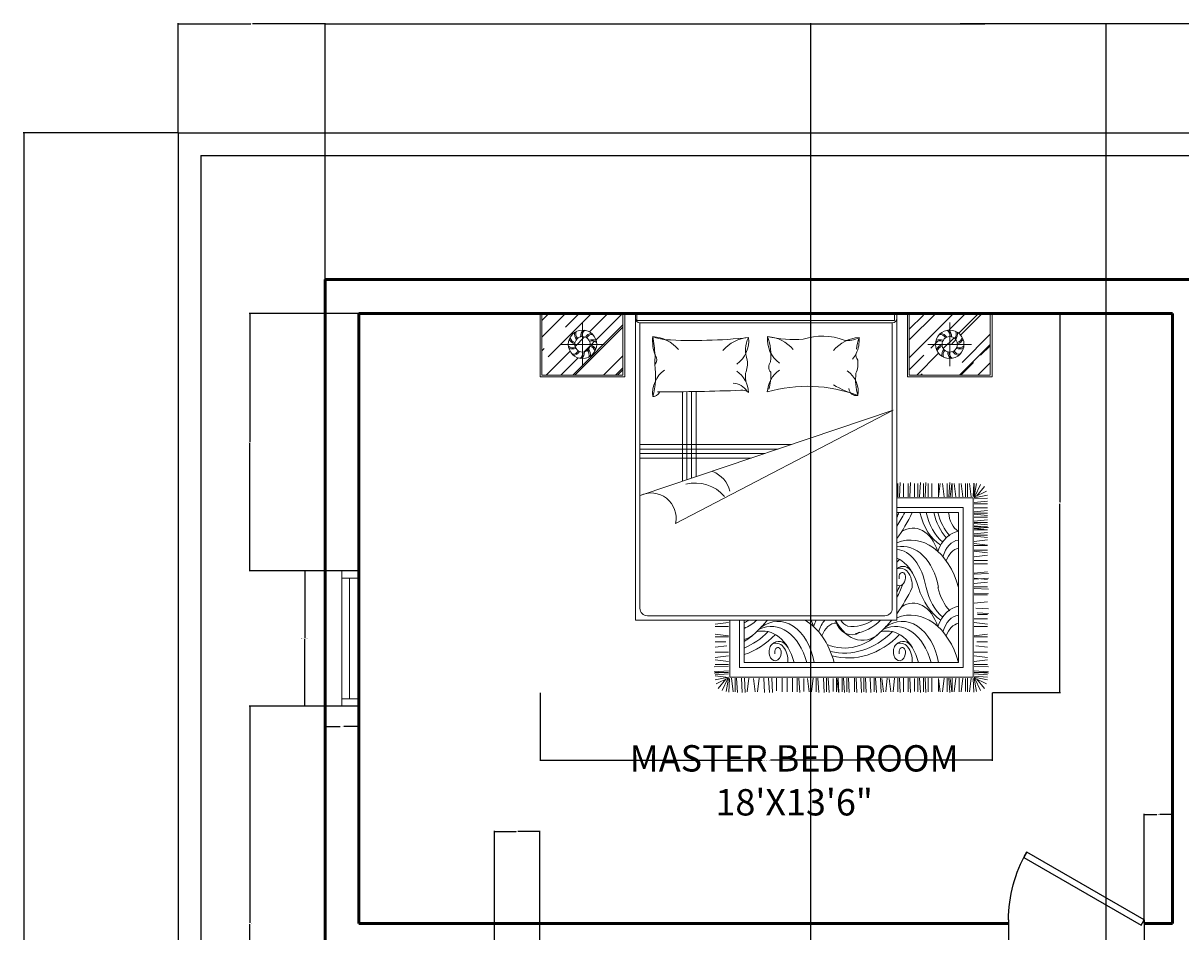
# Model space of a CAD drawing. Units: inches. Extents: x -28 to 483, y -584 to 51.
# Tile 5 of 6: x -28 to 279, y -191 to 51. Entities that reach past the tile are written whole.
import ezdxf

# ---------------------------------------------------------------- set-up
doc = ezdxf.new("R2010")
doc.units = ezdxf.units.IN
doc.header["$MEASUREMENT"] = 0
for name, color, linetype, lineweight in [('A-ANNO-DIMS', 2, 'Continuous', 18), ('A-AREA-IDEN', 7, 'Continuous', 25), ('A-DOOR', 4, 'Continuous', 25), ('A-FURN', 30, 'Continuous', 18), ('A-GLAZ', 5, 'Continuous', 18), ('A-WALL', 7, 'Continuous', 50), ('C-PROP', 7, 'Continuous', 25)]:
    doc.layers.add(name, color=color, linetype=linetype, lineweight=lineweight)
doc.styles.get("Standard").update_dxf_attribs({"font": 'arial.ttf'})
doc.dimstyles.get("Standard").update_dxf_attribs({"dimtxt": 0.18, "dimasz": 0.18, "dimexe": 0.18, "dimexo": 0.0625, "dimgap": 0.09, "dimtad": 0, "dimtih": 1, "dimtoh": 1, "dimdec": 4, "dimzin": 0, "dimdsep": 46, "dimtxsty": 'Standard', "dimcen": 0.09, "dimadec": 0, "dimazin": 0, "dimtfac": 1, "dimtdec": 4, "dimtofl": 0, "dimtmove": 0, "dimatfit": 3, "dimfxl": 1, "dimtolj": 1, "dimtzin": 0, "dimarcsym": 0})

# ---------------------------------------------------------------- blocks, each defined once
blk = doc.blocks.new('*U2')
for p, q in [((0, 0), (0, -6)), ((40, 0), (40, -6))]:
    blk.add_line(p, q)
blk.add_lwpolyline([(0, 0), (34.64, 20), (35.52, 18.48), (0.87, -1.52)], close=True)
blk.add_arc((0, 0), 40, 0, 30)
blk = doc.blocks.new('A$C64B41DC1')
for p, q in [((0, 2.5079), (2.9903, 2.5079)), ((0, 2.0879), (0, 2.5079)), ((0.012, 2.4618), (0.0581, 2.5079)), ((0.012, 2.3515), (0.1684, 2.5079)), ((0.012, 2.0999), (0.012, 2.5079)), ((0.0543, 2.2213), (0.3409, 2.5079)), ((0.1689, 2.4179), (0.2589, 2.5079)), ((0.3265, 2.386), (0.4484, 2.5079)), ((0.3699, 2.3332), (0.5445, 2.5079)), ((0.548, 2.5079), (0.548, 2.0999)), ((0.56, 2.5079), (0.56, 2.0879)), ((0.6301, 2.5079), (0.6301, 0.4779)), ((0.6401, 2.461), (0.6401, 2.5079)), ((0.6401, 2.5079), (2.344, 2.5079)), ((2.344, 2.461), (0.6401, 2.461)), ((2.344, 2.5079), (2.3601, 2.5079)), ((2.344, 2.5079), (2.344, 2.461)), ((2.3601, 2.5079), (2.3601, 2.4761)), ((2.3601, 0.4779), (2.3601, 2.5079)), ((2.4303, 2.5079), (2.4303, 2.0879)), ((2.4423, 2.5079), (2.4423, 2.0999)), ((2.4423, 2.3333), (2.6169, 2.5079)), ((2.4423, 2.2145), (2.7357, 2.5079)), ((2.4423, 2.404), (2.5354, 2.4971)), ((2.705, 2.398), (2.8149, 2.5079)), ((2.7691, 2.3772), (2.8998, 2.5079)), ((2.7819, 2.3646), (2.9252, 2.5079)), ((2.9783, 2.0999), (2.9783, 2.5079)), ((2.9903, 2.0879), (2.9903, 2.5079)), ((0.2157, 2.0999), (0.548, 2.4322)), ((0.2299, 2.0999), (0.548, 2.418)), ((0.2804, 2.1597), (0.2804, 2.4481)), ((0.6601, 2.4461), (1.4951, 2.4461)), ((0.6601, 2.4461), (0.6601, 0.5579)), ((1.4951, 2.4461), (0.6697, 2.4461)), ((2.3301, 2.4461), (1.4951, 2.4461)), ((2.3301, 0.5579), (2.3301, 2.4461)), ((2.7099, 2.1597), (2.7099, 2.4481)), ((0.1362, 2.3039), (0.4246, 2.3039)), ((0.2311, 2.2906), (0.2937, 2.3532)), ((0.3405, 2.3039), (0.3605, 2.3238)), ((2.8541, 2.3039), (2.5657, 2.3039)), ((2.5849, 2.2779), (2.6158, 2.3088)), ((2.6158, 2.3088), (2.6313, 2.3243)), ((2.6674, 2.2756), (2.7382, 2.3464)), ((2.7249, 2.3076), (2.7512, 2.3339)), ((2.7746, 2.0999), (2.9783, 2.3036)), ((2.7914, 2.1846), (2.9783, 2.3715)), ((0.012, 2.261), (0.0275, 2.2765)), ((0.0404, 2.0999), (0.1982, 2.2578)), ((0.2905, 2.2539), (0.3304, 2.2938)), ((0.4194, 2.0999), (0.548, 2.2285)), ((2.4423, 2.1353), (2.5382, 2.2312)), ((2.4918, 2.0999), (2.6366, 2.2447)), ((2.9144, 2.2312), (2.9783, 2.2951)), ((0.1365, 2.0999), (0.251, 2.2144)), ((0.4986, 2.0999), (0.548, 2.1493)), ((2.7831, 2.0999), (2.8678, 2.1846)), ((2.8962, 2.0999), (2.9783, 2.182)), ((0.56, 2.0879), (0, 2.0879)), ((0.548, 2.0999), (0.012, 2.0999)), ((0.5127, 2.0999), (0.548, 2.1352)), ((2.4303, 2.0879), (2.9903, 2.0879)), ((2.4423, 2.0999), (2.9783, 2.0999)), ((2.5172, 2.0999), (2.5269, 2.1096)), ((1.0315, 1.9916), (1.0315, 1.4279)), ((0.9415, 1.9902), (0.9415, 1.3975)), ((0.9715, 1.9906), (0.9715, 1.4076)), ((1.0015, 1.991), (1.0015, 1.4177)), ((2.3349, 1.8678), (0.6613, 1.3029)), ((0.8956, 1.1191), (2.3349, 1.8678)), ((1.6636, 1.6412), (0.6601, 1.6412)), ((1.5748, 1.6112), (0.6601, 1.6112)), ((2.3665, 1.295), (2.3665, 1.3839)), ((2.377, 1.295), (2.3822, 1.3891)), ((2.4032, 1.295), (2.4032, 1.3839)), ((2.4346, 1.295), (2.4346, 1.3839)), ((2.4451, 1.295), (2.4503, 1.3891)), ((2.4774, 1.2957), (2.4774, 1.3837)), ((2.5, 1.295), (2.5, 1.3839)), ((2.5105, 1.295), (2.5157, 1.3891)), ((2.5367, 1.295), (2.5367, 1.3839)), ((2.5471, 1.295), (2.5524, 1.3891)), ((2.5681, 1.295), (2.5681, 1.3839)), ((2.5918, 1.295), (2.5918, 1.3839)), ((2.6346, 1.2957), (2.6346, 1.3837)), ((2.6362, 1.2957), (2.6467, 1.3839)), ((2.6729, 1.295), (2.6624, 1.3839)), ((2.6938, 1.295), (2.6938, 1.3839)), ((2.7043, 1.295), (2.7095, 1.3891)), ((2.7127, 1.2957), (2.7232, 1.3839)), ((2.7253, 1.295), (2.7253, 1.3839)), ((2.7494, 1.295), (2.7389, 1.3839)), ((2.7718, 1.295), (2.7718, 1.3839)), ((2.7959, 1.295), (2.7854, 1.3839)), ((2.8146, 1.2957), (2.8146, 1.3837)), ((2.8146, 1.2957), (2.8146, 1.3837)), ((2.8282, 1.295), (2.8282, 1.3839)), ((2.8282, 1.295), (2.8282, 1.3839)), ((2.8523, 1.295), (2.8418, 1.3839)), ((2.8523, 1.295), (2.8418, 1.3839)), ((2.8653, 1.2966), (2.8688, 1.3861)), ((2.8711, 1.2957), (2.8711, 1.3837)), ((2.8711, 1.2957), (2.8875, 1.3822)), ((2.8713, 1.2927), (2.954, 1.3315)), ((2.8717, 1.2884), (2.9588, 1.3058)), ((2.8765, 1.2958), (2.9132, 1.3758)), ((2.8893, 1.3011), (2.9394, 1.3636)), ((2.3601, 1.2873), (2.8639, 1.2873)), ((2.8639, 1.2873), (2.8639, 0.1018)), ((2.8716, 1.2565), (2.9605, 1.2669)), ((2.8723, 1.2489), (2.9603, 1.2489)), ((2.8744, 1.2817), (2.9603, 1.2869)), ((2.3601, 1.2233), (2.7999, 1.2233)), ((2.3601, 1.1913), (2.7679, 1.1912)), ((2.7679, 1.1912), (2.7679, 0.1978)), ((2.7999, 1.2233), (2.7999, 0.1658)), ((2.8716, 1.2212), (2.9605, 1.2212)), ((2.8716, 1.1947), (2.9605, 1.2052)), ((2.8716, 1.181), (2.9605, 1.1705)), ((2.8716, 1.1595), (2.9605, 1.1595)), ((2.8723, 1.1872), (2.9603, 1.1872)), ((2.8716, 1.133), (2.9605, 1.1435)), ((2.8716, 1.1193), (2.9605, 1.1088)), ((2.8716, 1.1035), (2.9605, 1.093)), ((2.8716, 1.0965), (2.9605, 1.0965)), ((2.8716, 1.086), (2.9657, 1.0913)), ((2.8716, 1.0756), (2.9605, 1.0756)), ((2.8723, 1.1255), (2.9603, 1.1255)), ((2.8723, 1.0858), (2.9605, 1.0753)), ((2.8716, 1.0491), (2.9605, 1.0596)), ((2.8716, 1.0354), (2.9605, 1.0249)), ((2.8723, 1.0416), (2.9603, 1.0416)), ((2.8723, 0.9987), (2.9605, 1.0092)), ((2.8716, 0.9346), (2.9605, 0.9241)), ((2.8723, 0.985), (2.9605, 0.9745)), ((2.8723, 0.9735), (2.9603, 0.9735)), ((2.8723, 0.9408), (2.9603, 0.9408)), ((2.8723, 0.8979), (2.9605, 0.9084)), ((2.8723, 0.8726), (2.9603, 0.8726)), ((2.8723, 0.8505), (2.9603, 0.8505)), ((2.8716, 0.7885), (2.9605, 0.799)), ((2.8716, 0.7818), (2.9657, 0.787)), ((2.8716, 0.7503), (2.9657, 0.7556)), ((2.8716, 0.7204), (2.9605, 0.7309)), ((2.8716, 0.6995), (2.9605, 0.6995)), ((2.8723, 0.7571), (2.9605, 0.7466)), ((2.8716, 0.689), (2.9657, 0.6838)), ((2.8716, 0.6576), (2.9657, 0.6523)), ((2.8716, 0.6471), (2.9605, 0.6471)), ((2.8716, 0.5903), (2.9605, 0.6007)), ((2.882, 0.5582), (2.9657, 0.5536)), ((0.6301, 0.4779), (2.3601, 0.4779)), ((0.7101, 0.5079), (2.2801, 0.5079)), ((1.2465, 0.4625), (1.1576, 0.452)), ((1.2542, 0.1018), (1.2542, 0.4779)), ((1.3182, 0.1658), (1.3182, 0.4779)), ((1.3502, 0.1978), (1.3502, 0.4779)), ((2.8716, 0.4877), (2.9603, 0.4877)), ((2.8716, 0.4625), (2.9605, 0.452)), ((2.8909, 0.5263), (2.9657, 0.5222)), ((2.8928, 0.5169), (2.9605, 0.5169)), ((1.2465, 0.3746), (1.1576, 0.3851)), ((1.2465, 0.4365), (1.1577, 0.4365)), ((2.8716, 0.4365), (2.9603, 0.4365)), ((2.8716, 0.3746), (2.9605, 0.3851)), ((1.2355, 0.3092), (1.1576, 0.3)), ((1.2465, 0.3684), (1.1577, 0.3684)), ((1.2285, 0.3357), (1.1577, 0.3357)), ((2.8716, 0.3684), (2.9603, 0.3684)), ((2.8826, 0.3092), (2.9605, 0.3)), ((2.8896, 0.3357), (2.9603, 0.3357)), ((1.2457, 0.2423), (1.1576, 0.2319)), ((1.2457, 0.2676), (1.1577, 0.2676)), ((2.8723, 0.2676), (2.9603, 0.2676)), ((2.8723, 0.2423), (2.9605, 0.2319)), ((1.2465, 0.1742), (1.1524, 0.169)), ((1.2465, 0.2057), (1.1576, 0.2161)), ((1.2465, 0.1847), (1.1576, 0.1847)), ((2.7999, 0.1658), (1.3182, 0.1658)), ((2.7679, 0.1978), (1.3502, 0.1978)), ((2.8716, 0.2057), (2.9605, 0.2161)), ((2.8716, 0.1847), (2.9605, 0.1847)), ((2.8716, 0.1742), (2.9657, 0.169)), ((1.2465, 0.1428), (1.1524, 0.1376)), ((1.2465, 0.1334), (1.1524, 0.1281)), ((1.2465, 0.1323), (1.1576, 0.1323)), ((1.2465, 0.1323), (1.1576, 0.1323)), ((1.2465, 0.1), (1.1576, 0.1105)), ((1.2465, 0.1229), (1.1588, 0.1168)), ((1.2464, 0.1007), (1.1592, 0.0833)), ((1.2468, 0.0964), (1.1641, 0.0576)), ((1.2288, 0.088), (1.1787, 0.0255)), ((1.2415, 0.0933), (1.2049, 0.0133)), ((1.247, 0.0934), (1.2306, 0.0069)), ((1.2527, 0.0925), (1.2493, 0.003)), ((2.8639, 0.1018), (1.2542, 0.1018)), ((1.2658, 0.0941), (1.2762, 0.0052)), ((1.2899, 0.0941), (1.2899, 0.0052)), ((1.2999, 0.0941), (1.3051, 0)), ((1.3313, 0.0941), (1.3365, 0)), ((1.3523, 0.0941), (1.3575, 0)), ((1.3804, 0.0941), (1.3699, 0.0052)), ((1.4119, 0.0934), (1.4223, 0.0052)), ((1.4485, 0.0941), (1.438, 0.0052)), ((1.48, 0.0941), (1.4852, 0)), ((1.5114, 0.0941), (1.5166, 0)), ((1.5323, 0.0941), (1.5376, 0)), ((1.5638, 0.0941), (1.5638, 0.0105)), ((1.6021, 0.0941), (1.6021, 0.0052)), ((1.6336, 0.0941), (1.6336, 0.0052)), ((1.6702, 0.0941), (1.6702, 0.0052)), ((1.7017, 0.0941), (1.7017, 0.0052)), ((1.7122, 0.0941), (1.7174, 0)), ((1.7445, 0.0934), (1.7445, 0.0054)), ((1.7698, 0.0934), (1.7803, 0.0052)), ((1.8065, 0.0941), (1.796, 0.0052)), ((1.8274, 0.0941), (1.8274, 0.0052)), ((1.8379, 0.0941), (1.8431, 0)), ((1.8746, 0.0941), (1.8798, 0)), ((1.8955, 0.0941), (1.8955, 0.0052)), ((1.906, 0.0941), (1.9113, 0)), ((1.9384, 0.0934), (1.9384, 0.0054)), ((1.9609, 0.0941), (1.9609, 0.0052)), ((1.9636, 0.0934), (1.9741, 0.0052)), ((1.9714, 0.0941), (1.9766, 0)), ((1.9976, 0.0941), (1.9976, 0.0052)), ((2.0081, 0.0941), (2.0133, 0)), ((2.029, 0.0941), (2.029, 0.0052)), ((2.0395, 0.0941), (2.0447, 0)), ((2.0797, 0.0941), (2.0797, 0.0052)), ((2.0902, 0.0941), (2.0954, 0)), ((2.1216, 0.0941), (2.1269, 0)), ((2.1412, 0.0941), (2.1412, 0.0052)), ((2.1517, 0.0941), (2.1569, 0)), ((2.1831, 0.0941), (2.1884, 0)), ((2.2093, 0.0941), (2.2093, 0.0052)), ((2.2198, 0.0941), (2.225, 0)), ((2.2512, 0.0941), (2.2565, 0)), ((2.2603, 0.0934), (2.2707, 0.0052)), ((2.2969, 0.0941), (2.2864, 0.0052)), ((2.3089, 0.0934), (2.3193, 0.0052)), ((2.3455, 0.0941), (2.3351, 0.0052)), ((2.3665, 0.0941), (2.3665, 0.0052)), ((2.377, 0.0941), (2.3822, 0)), ((2.4032, 0.0941), (2.4032, 0.0052)), ((2.4346, 0.0941), (2.4346, 0.0052)), ((2.4451, 0.0941), (2.4503, 0)), ((2.4774, 0.0934), (2.4774, 0.0054)), ((2.5, 0.0941), (2.5, 0.0052)), ((2.5105, 0.0941), (2.5157, 0)), ((2.5367, 0.0941), (2.5367, 0.0052)), ((2.5471, 0.0941), (2.5524, 0)), ((2.5681, 0.0941), (2.5681, 0.0052)), ((2.5918, 0.0941), (2.5918, 0.0052)), ((2.6346, 0.0934), (2.6346, 0.0054)), ((2.6362, 0.0934), (2.6467, 0.0052)), ((2.6729, 0.0941), (2.6624, 0.0052)), ((2.6938, 0.0941), (2.6938, 0.0052)), ((2.7043, 0.0941), (2.7095, 0)), ((2.7127, 0.0934), (2.7232, 0.0052)), ((2.7253, 0.0941), (2.7253, 0.0052)), ((2.7494, 0.0941), (2.7389, 0.0052)), ((2.7718, 0.0941), (2.7718, 0.0052)), ((2.7959, 0.0941), (2.7854, 0.0052)), ((2.8146, 0.0934), (2.8146, 0.0054)), ((2.8282, 0.0941), (2.8282, 0.0052)), ((2.8523, 0.0941), (2.8418, 0.0052)), ((2.8653, 0.0925), (2.8688, 0.003)), ((2.8711, 0.0934), (2.8875, 0.0069)), ((2.8713, 0.0964), (2.954, 0.0576)), ((2.8716, 0.1428), (2.9657, 0.1376)), ((2.8716, 0.1334), (2.9657, 0.1281)), ((2.8716, 0.1323), (2.9605, 0.1323)), ((2.8716, 0.1229), (2.9593, 0.1168)), ((2.8717, 0.1007), (2.9588, 0.0833)), ((2.8744, 0.1074), (2.9603, 0.1022)), ((2.8765, 0.0933), (2.9132, 0.0133)), ((2.8893, 0.088), (2.9394, 0.0255))]:
    blk.add_line(p, q)
at = {"ltscale": 10}
for p, q in [((1.4859, 1.5812), (0.6601, 1.5812)), ((1.397, 1.5512), (0.6601, 1.5512))]:
    blk.add_line(p, q, dxfattribs=at)
for centre, radius in [((0.2804, 2.3039), 0.0942), ((2.7099, 2.3039), 0.0942), ((0.2804, 2.3039), 0.051), ((2.7099, 2.3039), 0.051)]:
    blk.add_circle(centre, radius)
for centre, radius, start, end in [((0.6601, 2.4761), 0.03, 180, 270), ((2.3301, 2.4761), 0.03, 270, 0), ((0.2887, 2.3745), 0.0605, 172.17003, 218.48975), ((0.2828, 2.3731), 0.0462, 160.30017, 220.53802), ((0.3286, 2.3561), 0.0605, 136.17003, 182.48975), ((0.3231, 2.3585), 0.0462, 124.30017, 184.53802), ((0.3501, 2.3178), 0.0605, 100.17003, 146.48975), ((2.6402, 2.3178), 0.0605, 33.51025, 79.82997), ((2.6672, 2.3585), 0.0462, 355.46198, 55.69983), ((2.6617, 2.3561), 0.0605, 357.51025, 43.82997), ((2.7075, 2.3731), 0.0462, 319.46198, 19.69983), ((2.7016, 2.3745), 0.0605, 321.51025, 7.82997), ((0.2457, 2.3659), 0.0605, 208.17003, 254.48975), ((0.2417, 2.3614), 0.0462, 196.30017, 256.53802), ((0.347, 2.323), 0.0462, 88.30017, 148.53802), ((0.3449, 2.2742), 0.0605, 64.17003, 110.48975), ((0.3455, 2.2802), 0.0462, 52.30017, 112.53802), ((0.3151, 2.2419), 0.0605, 28.17003, 74.48975), ((1.0526, 2.3302), 0.3085, 175.30484, 198.69419), ((-0.8702, 2.0941), 1.6364, 4.80985, 9.18918), ((0.8579, 2.6278), 0.2948, 247.51785, 264.26696), ((0.728, 2.111), 0.245, 40.4189, 85.9871), ((1.0164, 5.7096), 3.3803, 266.81337, 276.16021), ((1.3963, 2.1044), 0.245, 94.0129, 139.5811), ((1.1858, 2.3288), 0.1943, 306.5711, 5.88998), ((1.5348, 2.2652), 0.1767, 151.77364, 201.69827), ((1.6986, 2.3355), 0.1943, 174.11002, 233.4289), ((1.1481, 2.2311), 0.3783, 353.49469, 19.18669), ((1.6871, 3.192), 0.8561, 257.74383, 273.62843), ((1.4882, 2.111), 0.245, 40.4189, 85.9871), ((1.8674, 1.9709), 0.3878, 68.20259, 108.9817), ((2.1269, 2.1044), 0.245, 94.0129, 139.5811), ((2.0342, 2.4856), 0.1563, 261.59582, 298.90918), ((1.9165, 2.3288), 0.1943, 333.73715, 5.88998), ((2.6058, 2.2028), 0.517, 163.60457, 172.3273), ((2.6448, 2.2802), 0.0462, 67.46198, 127.69983), ((2.6454, 2.2742), 0.0605, 69.51025, 115.82997), ((2.6752, 2.2419), 0.0605, 105.51025, 151.82997), ((2.6433, 2.323), 0.0462, 31.46198, 91.69983), ((2.7486, 2.3614), 0.0462, 283.46198, 343.69983), ((2.7446, 2.3659), 0.0605, 285.51025, 331.82997), ((0.2153, 2.3276), 0.0462, 232.30017, 292.53802), ((0.2158, 2.3336), 0.0605, 244.17003, 290.48975), ((0.2138, 2.2848), 0.0462, 268.30017, 328.53802), ((0.2107, 2.29), 0.0605, 280.17003, 326.48975), ((0.2377, 2.2493), 0.0462, 304.30017, 4.53802), ((0.2322, 2.2517), 0.0605, 316.17003, 2.48975), ((0.2779, 2.2347), 0.0462, 340.30017, 40.53802), ((0.272, 2.2333), 0.0605, 352.17003, 38.48975), ((0.3191, 2.2464), 0.0462, 16.30017, 76.53802), ((0.7274, 2.2013), 0.0446, 314.4736, 42.17134), ((-1.6008, 2.277), 2.3618, 357.39054, 358.88764), ((1.9165, 2.3288), 0.1943, 320.94042, 333.73715), ((2.1347, 2.2313), 0.0459, 165.35061, 223.26844), ((2.6712, 2.2464), 0.0462, 103.46198, 163.69983), ((2.7182, 2.2333), 0.0605, 141.51025, 187.82997), ((2.7123, 2.2347), 0.0462, 139.46198, 199.69983), ((2.7581, 2.2517), 0.0605, 177.51025, 223.82997), ((2.7526, 2.2493), 0.0462, 175.46198, 235.69983), ((2.7796, 2.29), 0.0605, 213.51025, 259.82997), ((2.7765, 2.2848), 0.0462, 211.46198, 271.69983), ((2.7744, 2.3336), 0.0605, 249.51025, 295.82997), ((2.775, 2.3276), 0.0462, 247.46198, 307.69983), ((0.2688, 2.0945), 0.4956, 344.0243, 8.70709), ((1.204, 2.1778), 0.1681, 337.01697, 7.53676), ((1.5671, 2.1546), 0.0547, 142.08329, 220.902), ((1.9346, 2.1778), 0.1681, 337.01697, 7.53676), ((0.9385, 1.978), 0.1943, 126.5711, 185.88998), ((1.1858, 1.9714), 0.1943, 4.31813, 53.4289), ((1.5415, 2.0969), 0.1834, 175.22328, 196.23004), ((1.7059, 1.9714), 0.204, 127.11975, 175.09005), ((1.1965, 2.0983), 0.3299, 343.79543, 3.55541), ((1.9394, 1.991), 0.1651, 351.26213, 55.75721), ((2.4617, 2.0719), 0.3745, 173.82958, 196.4356), ((0.7246, 18.8439), 16.8552, 270.17399, 272.05214), ((1.2687, 1.9248), 0.1223, 33.62799, 86.47438), ((1.3401, 1.9404), 0.0603, 49.09906, 101.37023), ((1.7676, 1.0629), 0.9631, 69.65065, 105.96307), ((2.2748, 2.5795), 0.6373, 238.34989, 254.31375), ((2.0911, 2.0123), 0.0478, 179.77267, 283.80184), ((0.7417, 2.0149), 0.057, 273.47085, 328.54118), ((0.728, 2.2025), 0.245, 274.0129, 278.34166), ((1.0747, 1.2871), 0.1871, 14.1863, 69.12121), ((1.0274, 1.1334), 0.2527, 40.62904, 104.37123), ((0.7347, 1.1553), 0.1649, 347.31088, 116.44537), ((0.7101, 0.5579), 0.05, 180, 270), ((2.2801, 0.5579), 0.05, 270, 0)]:
    blk.add_arc(centre, radius, start, end)
for centre, major_axis, ratio, start_param, end_param in [((1.9938, 1.6262), (0, -0.7531), 0.68, 0.797284, 0.954936), ((2.0643, 1.466), (0, -0.5322), 0.68, 7.239912, 7.311536), ((1.9052, 1.7397), (0, -0.9842), 0.68, 0.74745, 0.979724), ((2.7455, 1.3081), (0, 0.3614), 0.68, 1.900046, 2.742661), ((2.7868, 1.3081), (0, 0.3614), 0.68, 1.900046, 2.614747), ((2.8372, 1.3081), (0, 0.3614), 0.68, 1.900046, 2.479658), ((2.8607, 1.3211), (0, 0.3614), 0.68, 1.938265, 2.479658), ((2.8057, 1.2079), (0, -0.1524), 0.68, 4.821745, 5.895886), ((2.4665, 0.8216), (0, -0.2664), 0.68, 2.006169, 3.565187), ((2.4513, 0.5069), (0, 0.502), 0.68, 5.095327, 6.553458), ((2.7862, 0.8069), (0, -0.2615), 0.68, 3.244645, 4.205018), ((2.7784, 0.8289), (0, -0.1802), 0.68, 3.227058, 4.318474), ((2.396, 0.6032), (0, 0.3641), 0.68, -1.3172, 0.145284), ((2.3507, 0.5642), (0.0073, 0.3819), 0.56205, -1.21172, -0.009991), ((2.7821, 0.7971), (0, -0.1589), 0.68, 3.272942, 4.229533), ((2.2964, 0.5771), (0, -0.3263), 0.68, 1.938944, 2.850232), ((2.0403, 1.6015), (0, -0.8763), 0.68, 6.849801, 6.887077), ((2.4005, 0.7132), (0, -0.1214), 0.68, 2.284368, 3.652258), ((2.3834, 0.7081), (0, 0.1147), 0.68, 4.593909, 6.585576), ((2.3961, 0.7628), (0, -0.0317), 0.68, 1.462497, 5.046281), ((2.3774, 0.7653), (0, -0.0593), 0.68, 5.841311, 7.755362), ((1.9938, 1.1295), (-0.0678, 0.7439), 0.610498, 3.917146, 4.063997), ((2.0643, 0.9693), (0, -0.5322), 0.68, 7.239912, 7.336618), ((1.9052, 1.243), (0, -0.9842), 0.68, 0.74745, 0.979724), ((2.7455, 0.8114), (-0.0599, 0.3735), 0.695517, 1.775813, 2.548612), ((2.7868, 0.8114), (0, 0.3614), 0.68, 1.900046, 2.614747), ((2.8607, 0.8243), (0, 0.3614), 0.68, 1.938265, 2.479658), ((2.4665, 0.3249), (0, -0.2664), 0.68, 2.006169, 3.565187), ((2.4513, 0.0102), (0, 0.502), 0.68, 5.095327, 6.553458), ((2.7862, 0.3102), (0, -0.2615), 0.68, 3.244645, 4.205018), ((1.242, 0.9693), (0, -0.5322), 0.68, 6.586764, 6.677612), ((1.1714, 1.1295), (-0.1157, 0.7241), 0.59432, 3.291697, 3.50733), ((1.0828, 1.243), (0, -0.9842), 0.68, 0.565948, 0.680366), ((1.5283, 0.0674), (0, -0.3703), 0.68, 1.930561, 3.464283), ((1.5736, 0.1065), (0, 0.3641), 0.68, -1.3172, 0.476403), ((1.6289, 0.0102), (0, 0.502), 0.68, 6.655152, 6.661293), ((1.6289, 0.0102), (0, 0.502), 0.68, 5.095327, 5.911219), ((1.6442, 0.3249), (0, -0.2664), 0.68, 2.006169, 2.182797), ((1.9638, 0.3102), (0, -0.2615), 0.68, 4.015924, 4.205018), ((1.956, 0.3322), (0, -0.1802), 0.68, 3.770744, 4.318474), ((2.0606, 0.5616), (0, -0.1803), 0.68, 5.194792, 5.929328), ((2.0606, 0.5616), (0, -0.1803), 0.68, 5.194792, 6.723255), ((2.1315, 0.6603), (0, -0.3155), 0.68, 5.328638, 6.949396), ((2.0549, 0.5656), (0, -0.1303), 0.68, 5.450951, 6.054641), ((2.0643, 0.9693), (0, -0.5322), 0.68, 6.20013, 6.677612), ((1.9938, 1.1295), (-0.0678, 0.7439), 0.610498, 3.199135, 3.592282), ((1.9052, 1.243), (0, -0.9842), 0.68, 0.565948, 0.680366), ((2.3507, 0.0674), (0, -0.3703), 0.68, 1.930561, 3.464283), ((2.396, 0.1065), (0, 0.3641), 0.68, -1.3172, 0.476403), ((2.4513, 0.0102), (0, 0.502), 0.68, 6.655152, 6.661293), ((2.7784, 0.3322), (0, -0.1802), 0.68, 3.227058, 4.318474), ((1.1933, 0.9181), (0, -0.624), 0.68, 0.378672, 0.625379), ((1.3091, 0.6603), (0, -0.3155), 0.68, 6.475719, 6.949396), ((1.1911, 1.1066), (0, 0.8458), 0.68, 3.421828, 3.728616), ((1.2179, 1.1047), (0, -0.8763), 0.68, 6.507006, 6.887077), ((1.474, 0.0804), (0, -0.3263), 0.68, 1.938944, 3.339184), ((1.9597, 0.3004), (0, -0.1589), 0.68, 3.14258, 4.229533), ((2.0157, 0.9181), (0, -0.624), 0.68, -0.280078, 0.625379), ((2.0135, 1.1066), (0, 0.8458), 0.68, 2.978727, 3.728616), ((2.0403, 1.1047), (0, -0.8763), 0.68, 6.099302, 6.887077), ((2.2964, 0.0804), (0, -0.3263), 0.68, 1.938944, 3.339184), ((2.7821, 0.3004), (0, -0.1589), 0.68, 3.272942, 4.229533), ((1.555, 0.2685), (0, -0.0593), 0.68, 3.732151, 7.755362), ((1.5781, 0.2165), (0, -0.1214), 0.68, 2.284368, 3.726131), ((1.561, 0.2114), (0, 0.1147), 0.68, 4.593909, 6.647252), ((2.3774, 0.2685), (0, -0.0593), 0.68, 3.732151, 7.755362), ((2.4005, 0.2165), (0, -0.1214), 0.68, 2.284368, 3.726131), ((2.3834, 0.2114), (0, 0.1147), 0.68, 4.593909, 6.647252), ((1.5737, 0.2661), (0, -0.0317), 0.68, 1.462497, 5.046281), ((2.3961, 0.2661), (0, -0.0317), 0.68, 1.462497, 5.046281)]:
    blk.add_ellipse(centre, major_axis=major_axis, ratio=ratio, start_param=start_param, end_param=end_param)
blk = doc.blocks.new('WIN-36IN')
for p, q in [((0, 9), (0, 0)), ((2, 9), (2, 4.5)), ((34, 6.5), (2, 6.5)), ((34, 9), (34, 4.5)), ((36, 9), (36, 0)), ((36, 4.5), (0, 4.5))]:
    blk.add_line(p, q)
blk = doc.blocks.new('*D11')
at = {"layer": 'A-ANNO-DIMS', "color": 0, "lineweight": -2, "transparency": 16777216}
for p, q in [((51.78, -94.91), (46.26, -94.91)), ((46.44, -95.09), (46.44, -112.72)), ((46.44, -130.73), (46.44, -113.09)), ((51.78, -130.91), (46.26, -130.91))]:
    blk.add_line(p, q, dxfattribs=at)
at = {"layer": 'A-ANNO-DIMS', "color": 0, "transparency": 16777216}
for points in [[(46.41, -95.09), (46.47, -95.09), (46.44, -94.91)], [(46.41, -130.73), (46.47, -130.73), (46.44, -130.91)]]:
    blk.add_solid(points, dxfattribs=at)
at = {"layer": 'Defpoints', "color": 0, "transparency": 16777216}
for p in [(51.84, -94.91), (46.44, -130.91), (51.84, -130.91)]:
    blk.add_point(p, dxfattribs=at)
at = {"layer": 'A-ANNO-DIMS', "color": 0, "transparency": 16777216, "insert": (46.44, -112.91), "char_height": 0.18, "attachment_point": 5}
blk.add_mtext('\\A1;WINDOW 36 TYP.', dxfattribs=at)
blk = doc.blocks.new('*D12')
at = {"layer": 'A-ANNO-DIMS', "color": 0, "lineweight": -2, "transparency": 16777216}
for p, q in [((51.84, -130.97), (51.84, -136.49)), ((60.84, -130.97), (60.84, -136.49)), ((52.02, -136.31), (55.88, -136.31)), ((60.66, -136.31), (56.8, -136.31))]:
    blk.add_line(p, q, dxfattribs=at)
at = {"layer": 'A-ANNO-DIMS', "color": 0, "transparency": 16777216}
for points in [[(52.02, -136.28), (52.02, -136.34), (51.84, -136.31)], [(60.66, -136.28), (60.66, -136.34), (60.84, -136.31)]]:
    blk.add_solid(points, dxfattribs=at)
at = {"layer": 'Defpoints', "color": 0, "transparency": 16777216}
for p in [(51.84, -130.91), (60.84, -130.91), (60.84, -136.31)]:
    blk.add_point(p, dxfattribs=at)
at = {"layer": 'A-ANNO-DIMS', "color": 0, "transparency": 16777216, "insert": (56.34, -136.31), "char_height": 0.18, "attachment_point": 5}
blk.add_mtext('\\A1;9 TYP.', dxfattribs=at)
blk = doc.blocks.new('*D13')
at = {"layer": 'A-ANNO-DIMS', "color": 0, "lineweight": -2, "transparency": 16777216}
for p, q in [((108.96, -127.31), (108.96, -145.43)), ((228.98, -127.31), (228.98, -145.43)), ((109.14, -145.25), (167.8, -145.25)), ((228.8, -145.25), (170.13, -145.25))]:
    blk.add_line(p, q, dxfattribs=at)
at = {"layer": 'A-ANNO-DIMS', "color": 0, "transparency": 16777216}
for points in [[(109.14, -145.22), (109.14, -145.28), (108.96, -145.25)], [(228.8, -145.22), (228.8, -145.28), (228.98, -145.25)]]:
    blk.add_solid(points, dxfattribs=at)
at = {"layer": 'Defpoints', "color": 0, "transparency": 16777216}
for p in [(108.96, -127.25), (228.98, -127.25), (228.98, -145.25)]:
    blk.add_point(p, dxfattribs=at)
at = {"layer": 'A-ANNO-DIMS', "color": 0, "transparency": 16777216, "insert": (168.97, -145.25), "char_height": 0.18, "attachment_point": 5}
blk.add_mtext('\\A1;BED SET 120 TYP.', dxfattribs=at)
blk = doc.blocks.new('*D14')
at = {"layer": 'A-ANNO-DIMS', "color": 0, "lineweight": -2, "transparency": 16777216}
for p, q in [((229.04, -26.59), (247.16, -26.59)), ((246.98, -26.77), (246.98, -76.74)), ((246.98, -127.07), (246.98, -77.1)), ((229.04, -127.25), (247.16, -127.25))]:
    blk.add_line(p, q, dxfattribs=at)
at = {"layer": 'A-ANNO-DIMS', "color": 0, "transparency": 16777216}
for points in [[(246.95, -26.77), (247.01, -26.77), (246.98, -26.59)], [(246.95, -127.07), (247.01, -127.07), (246.98, -127.25)]]:
    blk.add_solid(points, dxfattribs=at)
at = {"layer": 'Defpoints', "color": 0, "transparency": 16777216}
for p in [(228.98, -26.59), (246.98, -26.59), (228.98, -127.25)]:
    blk.add_point(p, dxfattribs=at)
at = {"layer": 'A-ANNO-DIMS', "color": 0, "transparency": 16777216, "insert": (246.98, -76.92), "char_height": 0.18, "attachment_point": 5}
blk.add_mtext('\\A1;101 TYP.', dxfattribs=at)
blk = doc.blocks.new('*D20')
at = {"layer": 'A-ANNO-DIMS', "color": 0, "lineweight": -2, "transparency": 16777216}
for p, q in [((12.78, 21.41), (-28.29, 21.41)), ((-28.11, 21.23), (-28.11, -266.41)), ((-28.11, -554.41), (-28.11, -266.77)), ((12.78, -554.59), (-28.29, -554.59))]:
    blk.add_line(p, q, dxfattribs=at)
at = {"layer": 'A-ANNO-DIMS', "color": 0, "transparency": 16777216}
for points in [[(-28.14, 21.23), (-28.08, 21.23), (-28.11, 21.41)], [(-28.14, -554.41), (-28.08, -554.41), (-28.11, -554.59)]]:
    blk.add_solid(points, dxfattribs=at)
at = {"layer": 'Defpoints', "color": 0, "transparency": 16777216}
for p in [(-28.11, 21.41), (12.84, 21.41), (12.84, -554.59)]:
    blk.add_point(p, dxfattribs=at)
at = {"layer": 'A-ANNO-DIMS', "color": 0, "transparency": 16777216, "insert": (-28.11, -266.59), "char_height": 0.18, "attachment_point": 5}
blk.add_mtext('\\A1;576', dxfattribs=at)
blk = doc.blocks.new('*D21')
at = {"layer": 'A-ANNO-DIMS', "color": 0, "lineweight": -2, "transparency": 16777216}
for p, q in [((51.84, -17.53), (51.84, 50.54)), ((52.02, 50.36), (227.07, 50.36)), ((402.66, 50.36), (227.61, 50.36)), ((402.84, -17.53), (402.84, 50.54))]:
    blk.add_line(p, q, dxfattribs=at)
at = {"layer": 'A-ANNO-DIMS', "color": 0, "transparency": 16777216}
for points in [[(52.02, 50.39), (52.02, 50.33), (51.84, 50.36)], [(402.66, 50.39), (402.66, 50.33), (402.84, 50.36)]]:
    blk.add_solid(points, dxfattribs=at)
at = {"layer": 'Defpoints', "color": 0, "transparency": 16777216}
for p in [(402.84, 50.36), (51.84, -17.59), (402.84, -17.59)]:
    blk.add_point(p, dxfattribs=at)
at = {"layer": 'A-ANNO-DIMS', "color": 0, "transparency": 16777216, "insert": (227.34, 50.36), "char_height": 0.18, "attachment_point": 5}
blk.add_mtext('\\A1;351', dxfattribs=at)
blk = doc.blocks.new('*D23')
at = {"layer": 'A-ANNO-DIMS', "color": 0, "lineweight": -2, "transparency": 16777216}
for p, q in [((12.84, 21.47), (12.84, 50.54)), ((13.02, 50.36), (32.12, 50.36)), ((51.66, 50.36), (32.56, 50.36)), ((51.84, -17.53), (51.84, 50.54))]:
    blk.add_line(p, q, dxfattribs=at)
at = {"layer": 'A-ANNO-DIMS', "color": 0, "transparency": 16777216}
for points in [[(13.02, 50.39), (13.02, 50.33), (12.84, 50.36)], [(51.66, 50.39), (51.66, 50.33), (51.84, 50.36)]]:
    blk.add_solid(points, dxfattribs=at)
at = {"layer": 'Defpoints', "color": 0, "transparency": 16777216}
for p in [(51.84, 50.36), (12.84, 21.41), (51.84, -17.59)]:
    blk.add_point(p, dxfattribs=at)
at = {"layer": 'A-ANNO-DIMS', "color": 0, "transparency": 16777216, "insert": (32.34, 50.36), "char_height": 0.18, "attachment_point": 5}
blk.add_mtext('\\A1;39', dxfattribs=at)
blk = doc.blocks.new('*D29')
at = {"layer": 'A-ANNO-DIMS', "color": 0, "lineweight": -2, "transparency": 16777216}
for p, q in [((269.35, -188.53), (269.35, -159.46)), ((269.53, -159.64), (272.72, -159.64)), ((276.66, -159.64), (273.47, -159.64)), ((276.84, -188.53), (276.84, -159.46))]:
    blk.add_line(p, q, dxfattribs=at)
at = {"layer": 'A-ANNO-DIMS', "color": 0, "transparency": 16777216}
for points in [[(269.53, -159.61), (269.53, -159.67), (269.35, -159.64)], [(276.66, -159.61), (276.66, -159.67), (276.84, -159.64)]]:
    blk.add_solid(points, dxfattribs=at)
at = {"layer": 'Defpoints', "color": 0, "transparency": 16777216}
for p in [(276.84, -159.64), (269.35, -188.59), (276.84, -188.59)]:
    blk.add_point(p, dxfattribs=at)
at = {"layer": 'A-ANNO-DIMS', "color": 0, "transparency": 16777216, "insert": (273.1, -159.64), "char_height": 0.18, "attachment_point": 5}
blk.add_mtext('\\A1;7.491', dxfattribs=at)
blk = doc.blocks.new('*D33')
at = {"layer": 'A-ANNO-DIMS', "color": 0, "lineweight": -2, "transparency": 16777216}
for p, q in [((60.78, -26.59), (31.71, -26.59)), ((31.89, -26.77), (31.89, -60.57)), ((31.89, -94.73), (31.89, -60.93)), ((60.78, -94.91), (31.71, -94.91))]:
    blk.add_line(p, q, dxfattribs=at)
at = {"layer": 'A-ANNO-DIMS', "color": 0, "transparency": 16777216}
for points in [[(31.86, -26.77), (31.92, -26.77), (31.89, -26.59)], [(31.86, -94.73), (31.92, -94.73), (31.89, -94.91)]]:
    blk.add_solid(points, dxfattribs=at)
at = {"layer": 'Defpoints', "color": 0, "transparency": 16777216}
for p in [(31.89, -26.59), (60.84, -26.59), (60.84, -94.91)]:
    blk.add_point(p, dxfattribs=at)
at = {"layer": 'A-ANNO-DIMS', "color": 0, "transparency": 16777216, "insert": (31.89, -60.75), "char_height": 0.18, "attachment_point": 5}
blk.add_mtext('\\A1;68.32', dxfattribs=at)
blk = doc.blocks.new('*D34')
at = {"layer": 'A-ANNO-DIMS', "color": 0, "lineweight": -2, "transparency": 16777216}
for p, q in [((60.78, -130.91), (31.71, -130.91)), ((31.89, -131.09), (31.89, -188.42)), ((31.89, -246.11), (31.89, -188.78)), ((60.78, -246.29), (31.71, -246.29))]:
    blk.add_line(p, q, dxfattribs=at)
at = {"layer": 'A-ANNO-DIMS', "color": 0, "transparency": 16777216}
for points in [[(31.86, -131.09), (31.92, -131.09), (31.89, -130.91)], [(31.86, -246.11), (31.92, -246.11), (31.89, -246.29)]]:
    blk.add_solid(points, dxfattribs=at)
at = {"layer": 'Defpoints', "color": 0, "transparency": 16777216}
for p in [(31.89, -130.91), (60.84, -130.91), (60.84, -246.29)]:
    blk.add_point(p, dxfattribs=at)
at = {"layer": 'A-ANNO-DIMS', "color": 0, "transparency": 16777216, "insert": (31.89, -188.6), "char_height": 0.18, "attachment_point": 5}
blk.add_mtext('\\A1;115.39', dxfattribs=at)
blk = doc.blocks.new('*D46')
at = {"layer": 'A-ANNO-DIMS', "color": 0, "lineweight": -2, "transparency": 16777216}
for p, q in [((180.84, -337.03), (180.84, 50.54)), ((181.02, 50.36), (219.68, 50.36)), ((259.11, 50.36), (220.46, 50.36)), ((259.29, -337.03), (259.29, 50.54))]:
    blk.add_line(p, q, dxfattribs=at)
at = {"layer": 'A-ANNO-DIMS', "color": 0, "transparency": 16777216}
for points in [[(181.02, 50.39), (181.02, 50.33), (180.84, 50.36)], [(259.11, 50.39), (259.11, 50.33), (259.29, 50.36)]]:
    blk.add_solid(points, dxfattribs=at)
at = {"layer": 'Defpoints', "color": 0, "transparency": 16777216}
for p in [(259.29, 50.36), (180.84, -337.09), (259.29, -337.09)]:
    blk.add_point(p, dxfattribs=at)
at = {"layer": 'A-ANNO-DIMS', "color": 0, "transparency": 16777216, "insert": (220.07, 50.36), "char_height": 0.18, "attachment_point": 5}
blk.add_mtext('\\A1;78.45', dxfattribs=at)
blk = doc.blocks.new('*D48')
at = {"layer": 'A-ANNO-DIMS', "color": 0, "lineweight": -2, "transparency": 16777216}
for p, q in [((96.84, -193.03), (96.84, -163.96)), ((97.02, -164.14), (102.63, -164.14)), ((108.66, -164.14), (103.05, -164.14)), ((108.84, -193.03), (108.84, -163.96))]:
    blk.add_line(p, q, dxfattribs=at)
at = {"layer": 'A-ANNO-DIMS', "color": 0, "transparency": 16777216}
for points in [[(97.02, -164.11), (97.02, -164.17), (96.84, -164.14)], [(108.66, -164.11), (108.66, -164.17), (108.84, -164.14)]]:
    blk.add_solid(points, dxfattribs=at)
at = {"layer": 'Defpoints', "color": 0, "transparency": 16777216}
for p in [(108.84, -164.14), (96.84, -193.09), (108.84, -193.09)]:
    blk.add_point(p, dxfattribs=at)
at = {"layer": 'A-ANNO-DIMS', "color": 0, "transparency": 16777216, "insert": (102.84, -164.14), "char_height": 0.18, "attachment_point": 5}
blk.add_mtext('\\A1;12', dxfattribs=at)

msp = doc.modelspace()

# ---------------------------------------------------------------- linework, layer by layer
at = {"layer": 'A-WALL'}
for p, q in [((51.8432, -17.5877), (402.8432, -17.5877)), ((51.8432, -17.5877), (51.8432, -494.5877)), ((60.8432, -26.5877), (276.8432, -26.5877)), ((60.8432, -26.5877), (60.8432, -188.5877)), ((276.8432, -26.5877), (276.8432, -188.5877)), ((60.8432, -188.5877), (233.3523, -188.5877)), ((269.3523, -188.5877), (276.8432, -188.5877))]:
    msp.add_line(p, q, dxfattribs=at)
at = {"layer": 'C-PROP'}
for p, q in [((12.8432, 21.4123), (444.8432, 21.4123)), ((12.8432, 21.4123), (12.8432, -554.5877)), ((18.8432, 15.4123), (438.8432, 15.4123)), ((18.8432, 15.4123), (18.8432, -548.5877))]:
    msp.add_line(p, q, dxfattribs=at)

# ---------------------------------------------------------------- block references
at = {"layer": 'A-DOOR', "xscale": -0.9, "yscale": 0.9, "zscale": 0.9}
msp.add_blockref('*U2', (269.3523, -187.6877), dxfattribs=at)
at = {"layer": 'A-FURN', "xscale": 40.13733178260718, "yscale": 40.13733178260718, "zscale": 40.13733178260718}
msp.add_blockref('A$C64B41DC1', (108.9555, -127.2482), dxfattribs=at)
at = {"layer": 'A-GLAZ', "rotation": 269.9999999999999}
msp.add_blockref('WIN-36IN', (51.8428, -94.9071), dxfattribs=at)

# ---------------------------------------------------------------- texts
at = {"layer": 'A-AREA-IDEN', "insert": (125.7041, -141.2503), "char_height": 7, "attachment_point": 1}
msp.add_mtext_dynamic_manual_height_columns('\\pxqc;MASTER BED ROOM\\P18\'X13\'6"', width=101.426885, gutter_width=1, heights=[0], dxfattribs=at)

# ---------------------------------------------------------------- dimensions: what is measured, and where the dimension line sits
at = {"layer": 'A-ANNO-DIMS'}
for base, p1, p2, override, picture, middle in [((51.8432, 50.3623), (12.8432, 21.4123), (51.8432, -17.5877), {"dimdec": 0, "dimlfac": 1, "dimrnd": 0, "dimzin": 0, "dimdsep": 46, "dimlunit": 2}, '*D23', (32.3432, 50.3623)), ((402.8432, 50.3623), (51.8432, -17.5877), (402.8432, -17.5877), {"dimdec": 0, "dimlfac": 1, "dimrnd": 0, "dimzin": 0, "dimdsep": 46, "dimlunit": 2}, '*D21', (227.3432, 50.3623)), ((259.2944, 50.3623), (180.8432, -337.0877), (259.2944, -337.0877), {"dimdec": 2, "dimlfac": 1, "dimrnd": 0, "dimzin": 0, "dimdsep": 46, "dimlunit": 2}, '*D46', (220.0688, 50.3623)), ((276.8432, -159.6377), (269.3523, -188.5877), (276.8432, -188.5877), {"dimdec": 3, "dimlfac": 1, "dimrnd": 0, "dimzin": 0, "dimdsep": 46, "dimlunit": 2}, '*D29', (273.0977, -159.6377)), ((108.8432, -164.1377), (96.8432, -193.0877), (108.8432, -193.0877), {"dimdec": 0, "dimlfac": 1, "dimrnd": 0, "dimzin": 0, "dimdsep": 46, "dimlunit": 2}, '*D48', (102.8432, -164.1377))]:
    dim = msp.add_linear_dim(base=base, p1=p1, p2=p2, dimstyle='Standard', override=override, dxfattribs=at)
    dim.commit()
    dim.dimension.update_dxf_attribs({"geometry": picture, "text_midpoint": middle})
for base, p1, p2, override, picture, middle in [((-28.1068, 21.4123), (12.8432, -554.5877), (12.8432, 21.4123), {"dimdec": 0, "dimlfac": 1, "dimrnd": 0, "dimzin": 0, "dimdsep": 46, "dimlunit": 2}, '*D20', (-28.1068, -266.5877)), ((31.8932, -26.5877), (60.8432, -94.9071), (60.8432, -26.5877), {"dimdec": 2, "dimlfac": 1, "dimrnd": 0, "dimzin": 0, "dimdsep": 46, "dimlunit": 2}, '*D33', (31.8932, -60.7474)), ((31.8932, -130.9071), (60.8432, -246.2923), (60.8432, -130.9071), {"dimdec": 2, "dimlfac": 1, "dimrnd": 0, "dimzin": 0, "dimdsep": 46, "dimlunit": 2}, '*D34', (31.8932, -188.5997))]:
    dim = msp.add_linear_dim(base=base, p1=p1, p2=p2, angle=90, dimstyle='Standard', override=override, dxfattribs=at)
    dim.commit()
    dim.dimension.update_dxf_attribs({"geometry": picture, "text_midpoint": middle})
for base, p1, p2, angle, text, picture, middle in [((246.9805, -26.5877), (228.9772, -127.2482), (228.9772, -26.5877), 90, '<> TYP.', '*D14', (246.9805, -76.918)), ((46.4432, -130.9071), (51.8432, -94.9071), (51.8432, -130.9071), 270, 'WINDOW <> TYP.', '*D11', (46.4432, -112.9071))]:
    dim = msp.add_linear_dim(base=base, p1=p1, p2=p2, angle=angle, text=text, dimstyle='Standard', override={"dimdec": 0, "dimlfac": 1, "dimrnd": 0, "dimzin": 0, "dimdsep": 46, "dimlunit": 2}, dxfattribs=at)
    dim.commit()
    dim.dimension.update_dxf_attribs({"geometry": picture, "text_midpoint": middle})
for base, p1, p2, text, picture, middle in [((228.9772, -145.2515), (108.9555, -127.2482), (228.9772, -127.2482), 'BED SET <> TYP.', '*D13', (168.9664, -145.2515)), ((60.8432, -136.3071), (51.8432, -130.9071), (60.8432, -130.9071), '<> TYP.', '*D12', (56.3432, -136.3071))]:
    dim = msp.add_linear_dim(base=base, p1=p1, p2=p2, text=text, dimstyle='Standard', override={"dimdec": 0, "dimlfac": 1, "dimrnd": 0, "dimzin": 0, "dimdsep": 46, "dimlunit": 2}, dxfattribs=at)
    dim.commit()
    dim.dimension.update_dxf_attribs({"geometry": picture, "text_midpoint": middle})

doc.saveas('drawing.dxf')
